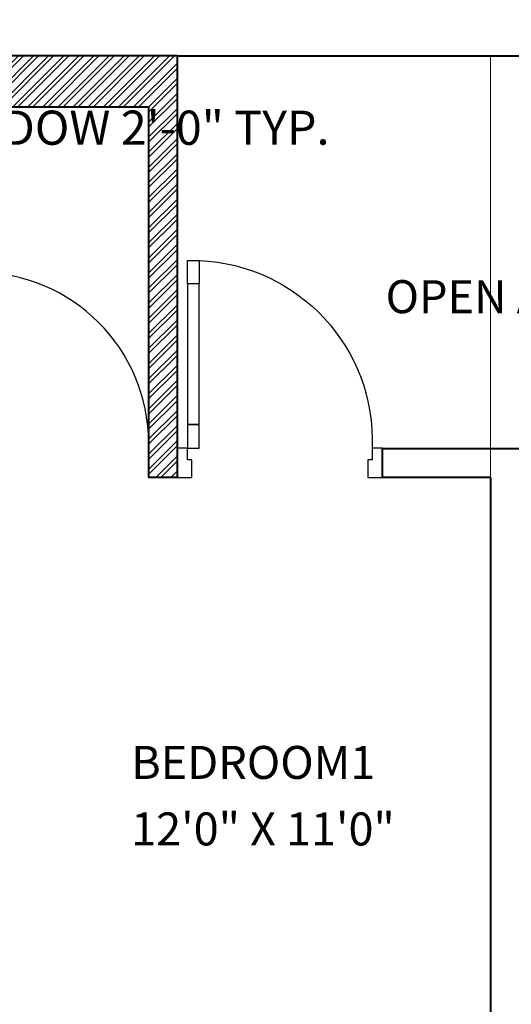
# Model space of a CAD drawing. Units: inches. Extents: x 528 to 2520, y -151 to 1354.
# Tile 35 of 41: x 2228 to 2315, y 731 to 904. Entities that reach past the tile are written whole.
import ezdxf

# ---------------------------------------------------------------- set-up
doc = ezdxf.new("R2010")
doc.units = ezdxf.units.IN
doc.header["$MEASUREMENT"] = 0
for name, color, linetype, lineweight in [('A-ANNO-DIMS', 2, 'Continuous', 18), ('A-AREA-IDEN', 7, 'Continuous', 18), ('A-Door', 150, 'Continuous', 25), ('A-ELEV-PROJ', 8, 'Continuous', 13), ('A-WALL-PATT', 6, 'Continuous', 13), ('walls', 7, 'Continuous', 40)]:
    doc.layers.add(name, color=color, linetype=linetype, lineweight=lineweight)
doc.layers.add('NT', color=1, linetype='Continuous')
doc.styles.get("Standard").update_dxf_attribs({"font": 'arial.ttf'})
doc.dimstyles.get("Standard").update_dxf_attribs({"dimtxt": 6, "dimasz": 2, "dimexe": 0.18, "dimexo": 0.0625, "dimgap": 0.09, "dimtad": 0, "dimtih": 1, "dimtoh": 1, "dimdec": 1, "dimzin": 0, "dimdsep": 46, "dimlunit": 3, "dimtxsty": 'Standard', "dimblk": 'ARCHTICK', "dimcen": 0.09, "dimadec": 0, "dimazin": 0, "dimtfac": 1, "dimtdec": 1, "dimtofl": 0, "dimtmove": 0, "dimatfit": 3, "dimfxl": 1, "dimtolj": 1, "dimtzin": 0, "dimarcsym": 0})

# ---------------------------------------------------------------- blocks, each defined once
blk = doc.blocks.new('A$C7DB75F4D')
at = {"layer": 'A-Door'}
for points in [[(625, 740), (625, 660), (665, 660), (665, 740)], [(625, 180), (625, 660), (665, 660), (665, 180)], [(625, 100), (625, 180), (665, 180), (665, 100)], [(35, 100), (35, 60), (50, 60), (50, 50), (50, 0), (0, 0), (0, 100)], [(665, 100), (700, 100), (700, 0), (650, 0), (650, 50), (650, 60), (665, 60)]]:
    blk.add_lwpolyline(points, close=True, dxfattribs=at)
at = {"layer": 'NT'}
blk.add_arc((650, 125), 615.5, 92.3278, 182.3278, dxfattribs=at)
blk = doc.blocks.new('DOOR-SWING-30')
for p, q in [((0, 6), (0, 0)), ((30, 6), (30, 0))]:
    blk.add_line(p, q)
blk.add_lwpolyline([(0, 6), (0, 36), (1.75, 36), (1.75, 6)], close=True)
blk.add_arc((0, 6), 30, 0, 90)
blk = doc.blocks.new('_ArchTick')
at = {"color": 0, "linetype": 'ByBlock', "const_width": 0.15}
blk.add_lwpolyline([(-0.5, -0.5), (0.5, 0.5)], dxfattribs=at)
blk = doc.blocks.new('*D56')
at = {"layer": 'A-ANNO-DIMS', "color": 0, "lineweight": -2, "transparency": 16777216}
for p, q in [((2167.01, 888.88), (2167.01, 885.16)), ((2191.01, 888.88), (2191.01, 885.16)), ((2167.01, 885.34), (2191.01, 885.34)), ((2191.01, 885.34), (2193.01, 885.34))]:
    blk.add_line(p, q, dxfattribs=at)
at = {"layer": 'Defpoints', "color": 0, "transparency": 16777216}
for p in [(2167.01, 888.94), (2191.01, 888.94), (2191.01, 885.34)]:
    blk.add_point(p, dxfattribs=at)
at = {"layer": 'A-ANNO-DIMS', "color": 0, "lineweight": -2, "transparency": 16777216, "xscale": 2, "yscale": 2, "zscale": 2, "rotation": 180}
blk.add_blockref('_ArchTick', (2167.01, 885.34), dxfattribs=at)
at = {"layer": 'A-ANNO-DIMS', "color": 0, "lineweight": -2, "transparency": 16777216, "xscale": 2, "yscale": 2, "zscale": 2}
blk.add_blockref('_ArchTick', (2191.01, 885.34), dxfattribs=at)
at = {"layer": 'A-ANNO-DIMS', "color": 0, "transparency": 16777216, "insert": (2239.21, 885.34), "char_height": 6, "attachment_point": 5}
blk.add_mtext('\\A1;WC WINDOW 2\'-0" TYP.', dxfattribs=at)

msp = doc.modelspace()

# ---------------------------------------------------------------- hatches: boundary and pattern name
at = {"layer": 'A-WALL-PATT'}
h = msp.add_hatch(dxfattribs=at)
h.set_pattern_fill('ANSI32', color=256, scale=5)
h.set_pattern_definition([(45, (1571.3155, -419.1643), (-1.3258252, 1.3258252), []), (45, (1572.1993, -419.1643), (-1.3258252, 1.3258252), [])])
h.paths.add_polyline_path([(2167.01, 744.69), (2158.01, 744.69), (2158.01, 549.94), (2169.56, 549.94), (2174.56, 549.94), (2174.56, 554.94), (2167.01, 554.94), (2167.01, 662.94), (2263.01, 662.94), (2263.01, 667.94), (2263.01, 686.94), (2269.01, 686.94), (2269.01, 691.94), (2258.01, 691.94), (2258.01, 667.94), (2167.01, 667.94)])
h.paths.add_polyline_path([(2260.02, 554.94), (2222.56, 554.94), (2222.56, 549.94), (2260.02, 549.94)])
h.paths.add_polyline_path([(2457.01, 752.2), (2448.01, 752.2), (2448.01, 691.94), (2358.01, 691.94), (2358.01, 686.94), (2448.01, 686.94), (2448.01, 554.94), (2358.01, 554.94), (2358.01, 549.94), (2448.01, 549.94), (2448.01, 405.94), (2406.01, 405.94), (2406.01, 396.94), (2457.01, 396.94)])
h.paths.add_polyline_path([(2457.01, 897.94), (2447.97, 897.94), (2447.97, 888.94), (2448.01, 888.94), (2448.01, 828.94), (2394.01, 828.94), (2394.01, 823.94), (2448.01, 823.94), (2448.01, 800.2), (2457.01, 800.2)])
h.paths.add_polyline_path([(2423.97, 897.94), (2359.01, 897.94), (2359.01, 828.94), (2355.58, 828.94), (2355.58, 823.94), (2364.01, 823.94), (2364.01, 829.94), (2364.01, 888.94), (2423.97, 888.94)])
h.paths.add_polyline_path([(2256.01, 897.94), (2191.01, 897.94), (2191.01, 888.94), (2251.01, 888.94), (2251.01, 828.94), (2251.01, 823.94), (2256.01, 823.94), (2256.01, 829.08)])
h.paths.add_polyline_path([(2167.01, 888.94), (2167.01, 897.94), (2158.01, 897.94), (2158.01, 792.69), (2167.01, 792.69), (2167.01, 823.94), (2221.01, 823.94), (2221.01, 828.94), (2167.01, 828.94)])
h.paths.add_polyline_path([(2316.01, 549.94), (2316.01, 554.94), (2296.02, 554.94), (2296.02, 549.94), (2311.01, 549.94), (2311.01, 455.12), (2316.01, 455.12)])
h.paths.add_polyline_path([(2311.01, 549.94), (2299.01, 549.94), (2299.01, 545.95), (2302.05, 545.95), (2302.05, 542.51), (2305.75, 542.51), (2305.75, 538.08), (2311.01, 538.08)], flags=17)
h.paths.add_polyline_path([(2358.01, 405.94), (2316.01, 405.94), (2316.01, 413.12), (2311.01, 413.12), (2311.01, 396.94), (2358.01, 396.94)])

# ---------------------------------------------------------------- linework, layer by layer
at = {"layer": 'A-ELEV-PROJ'}
msp.add_line((2311.01, 360.94), (2311.01, 897.94), dxfattribs=at)
at = {"layer": 'walls'}
for p, q in [((2256.01, 897.94), (2158.01, 897.94)), ((2256.01, 897.94), (2256.01, 828.94)), ((2256.01, 897.94), (2359.01, 897.94)), ((2251.01, 888.94), (2167.01, 888.94)), ((2251.01, 888.94), (2251.01, 828.94)), ((2251.01, 828.94), (2251.01, 823.94)), ((2256.01, 828.94), (2256.01, 823.94)), ((2359.01, 828.94), (2292.01, 828.94)), ((2292.01, 828.94), (2292.01, 823.94)), ((2256.01, 823.94), (2251.01, 823.94)), ((2311.01, 823.94), (2292.01, 823.94)), ((2311.01, 823.94), (2311.01, 691.94))]:
    msp.add_line(p, q, dxfattribs=at)

# ---------------------------------------------------------------- block references
at = {"layer": 'A-Door', "xscale": -0.0514539602427209, "yscale": 0.0514539602427209, "zscale": 0.0514539602427209}
msp.add_blockref('A$C7DB75F4D', (2292.03, 823.94), dxfattribs=at)
at = {"layer": 'A-Door'}
msp.add_blockref('DOOR-SWING-30', (2221.01, 823.94), dxfattribs=at)

# ---------------------------------------------------------------- texts
at = {"layer": 'A-AREA-IDEN'}
for s, height, p in [('OPEN AREA', 5.793, (2292.6, 852.77)), ('BEDROOM1 ', 5.793, (2247.95, 770.98)), ('12\'0" X 11\'0"', 5.7926, (2247.95, 759.3))]:
    msp.add_text(s, height=height, dxfattribs=at).set_placement(p)

# ---------------------------------------------------------------- dimensions: what is measured, and where the dimension line sits
at = {"layer": 'A-ANNO-DIMS'}
dim = msp.add_linear_dim(base=(2191.01, 885.34), p1=(2167.01, 888.94), p2=(2191.01, 888.94), text='WC WINDOW <> TYP.', dimstyle='Standard', override={"dimdec": 1, "dimlfac": 1, "dimrnd": 0, "dimzin": 1, "dimdsep": 46, "dimlunit": 4, "dimfrac": 2}, dxfattribs=at)
dim.commit()
dim.dimension.update_dxf_attribs({"geometry": '*D56', "text_midpoint": (2239.21, 885.34)})

doc.saveas('drawing.dxf')
